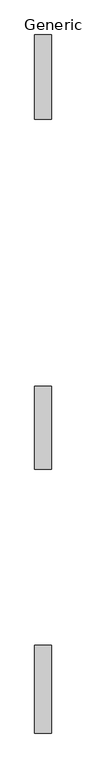
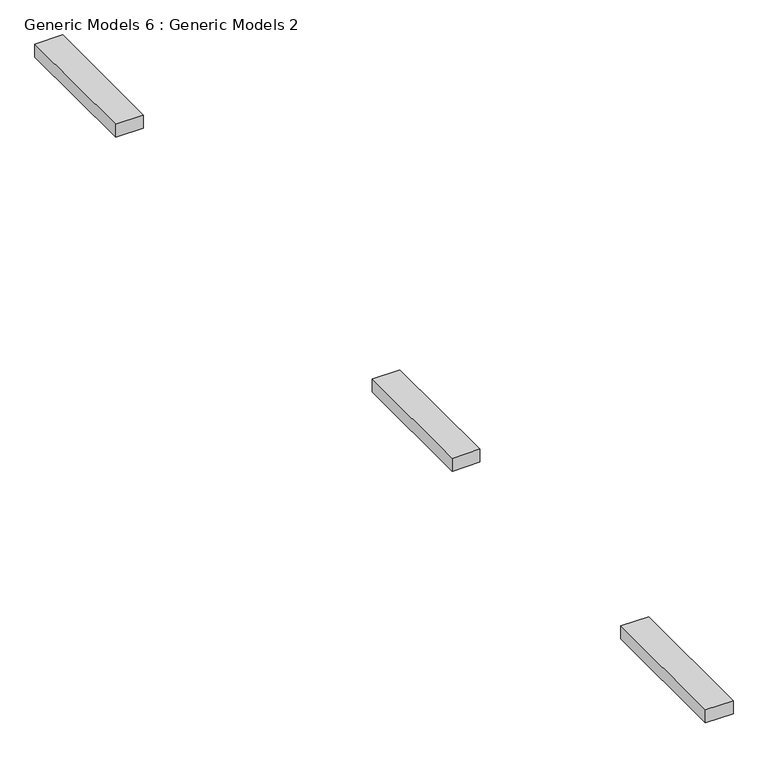
"""IFC4 building model written with IfcOpenShell, lengths in millimetres: proxy geometry, Generic Models 6 : Generic Models 2."""

from ifc_helpers import new_model, si_unit, frame, origin, place, context, project, spatial, polyline, outline, extrude, source, transform, mapped, element, save


def generic_models_6_generic_models_2_9348183e(model_context):
    return source(origin(), model_context, "Body", "SweptSolid", [
        extrude(outline(polyline([(-3150.8771954, -3782.7227897), (-3150.8771954, -5395.5736261), (-3455.6771954, -5395.5736261), (-3455.6771954, -3782.7227897), (-3150.8771954, -3782.7227897)])), frame((0.0, 0.0, 5613.4), z_axis=(0.0, 0.0, 1.0), x_axis=(1.0, 0.0, 0.0)), (0.0, 0.0, 1.0), 152.4),
        extrude(outline(polyline([(-3150.8771954, 963.3008967), (-3150.8771954, -560.9825441), (-3455.6771954, -560.9825441), (-3455.6771954, 963.3008967), (-3150.8771954, 963.3008967)])), frame((0.0, 0.0, 5613.4), z_axis=(0.0, 0.0, 1.0), x_axis=(1.0, 0.0, 0.0)), (0.0, 0.0, 1.0), 152.4),
        extrude(outline(polyline([(-3150.8771954, 7403.0267346), (-3150.8771954, 5859.3819001), (-3455.6771954, 5859.3819001), (-3455.6771954, 7403.0267346), (-3150.8771954, 7403.0267346)])), frame((0.0, 0.0, 5613.4), z_axis=(0.0, 0.0, 1.0), x_axis=(1.0, 0.0, 0.0)), (0.0, 0.0, 1.0), 152.4),
    ])


if __name__ == "__main__":
    model = new_model("IFC4")
    model_context = context("Model", 3, world=origin())
    ifc_project = project(units=[si_unit("LENGTHUNIT", "METRE", prefix="MILLI")], contexts=[model_context])
    site = spatial("IfcSite", under=ifc_project)
    building = spatial("IfcBuilding", under=site)
    placement = place(None, origin())
    generic_models_6_generic_models_2_shape = generic_models_6_generic_models_2_9348183e(model_context)
    element("IfcBuildingElementProxy", 1, Name="Generic Models 6 : Generic Models 2", ObjectType="Generic Models 6 : Generic Models 2", at=placement, inside=building, context=model_context, shape_type="MappedRepresentation", body=[
        mapped(generic_models_6_generic_models_2_shape, transform((0.0, 0.0, 0.0), x_axis=(1.0, 0.0, 0.0), y_axis=(0.0, 1.0, 0.0), z_axis=(0.0, 0.0, 1.0))),
    ])
    save(model, "model.ifc")
